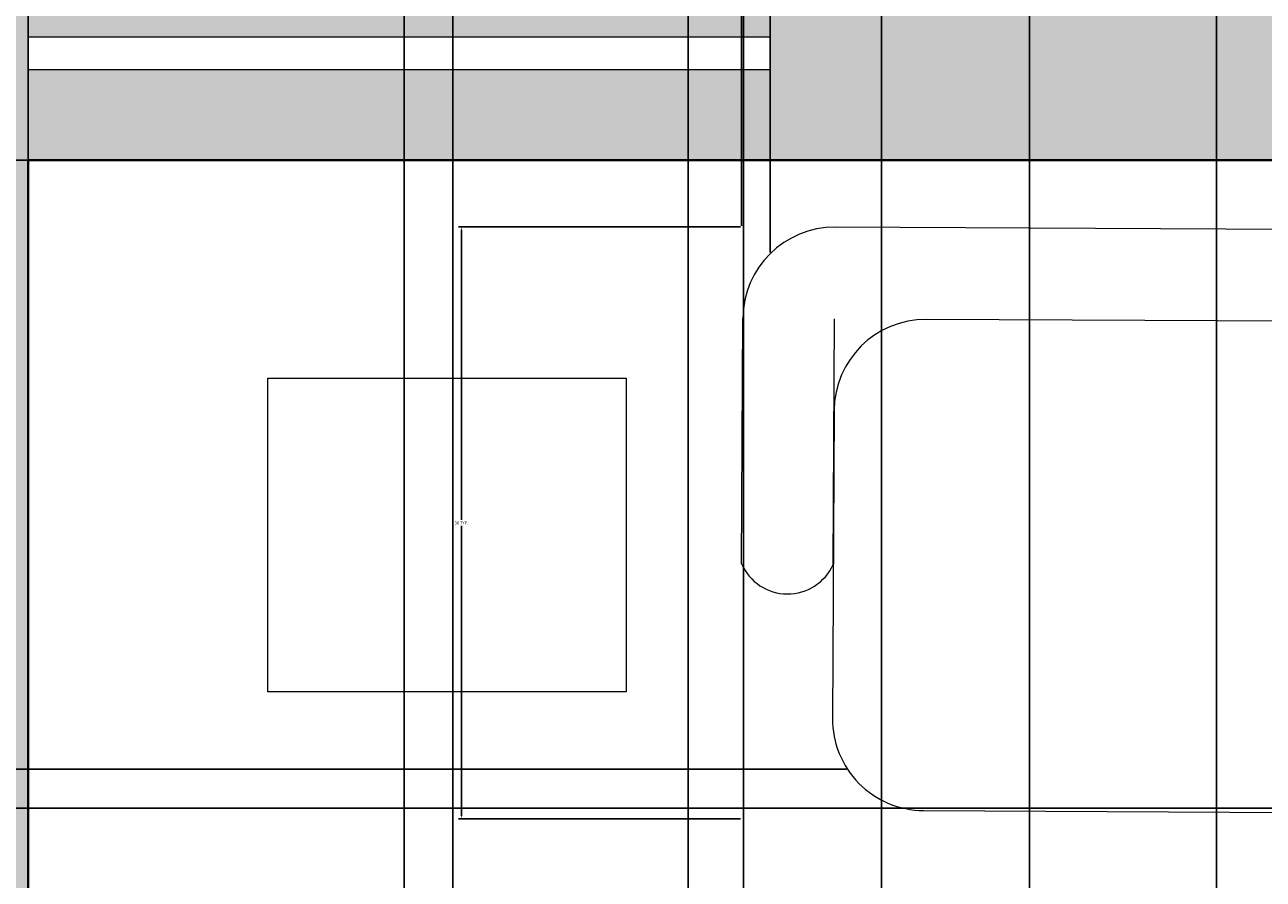
# Model space of a CAD drawing. Units: inches. Extents: x 818 to 1898, y 976 to 2364.
# Tile 28 of 96: x 1207 to 1282, y 1643 to 1695. Entities that reach past the tile are written whole.
import ezdxf

# ---------------------------------------------------------------- set-up
doc = ezdxf.new("R2010")
doc.units = ezdxf.units.IN
doc.header["$LTSCALE"] = 5
doc.header["$MEASUREMENT"] = 0
for name, color, linetype, lineweight in [('A-ANNO-DIMS', 2, 'Continuous', 18), ('A-FURN', 8, 'Continuous', 18), ('A-GLAZ', 4, 'Continuous', 18), ('A-WALL', 7, 'Continuous', 40)]:
    doc.layers.add(name, color=color, linetype=linetype, lineweight=lineweight)
doc.layers.add('A-GLAZ-PATT', color=141, linetype='Continuous', lineweight=9, true_color=0xadddf7)
doc.layers.add('A-WALL-PATT', color=251, linetype='Continuous', lineweight=13, true_color=0x636466)
doc.styles.get("Standard").update_dxf_attribs({"font": 'arial.ttf'})
doc.dimstyles.get("Standard").update_dxf_attribs({"dimtxt": 0.18, "dimasz": 0.18, "dimexe": 0.18, "dimexo": 0.0625, "dimgap": 0.09, "dimtad": 0, "dimtih": 1, "dimtoh": 1, "dimdec": 4, "dimzin": 0, "dimdsep": 46, "dimtxsty": 'Standard', "dimcen": 0.09, "dimadec": 0, "dimazin": 0, "dimtfac": 1, "dimtdec": 4, "dimtofl": 0, "dimtmove": 0, "dimatfit": 3, "dimfxl": 1, "dimtolj": 1, "dimtzin": 0, "dimarcsym": 0})

# ---------------------------------------------------------------- blocks, each defined once
blk = doc.blocks.new('SOFA-3-SEAT')
for p, q in [((39.87, 35.861), (5.697, 36.046)), ((0, 15.523), (0.081, 30.49)), ((5.586, 15.492), (5.667, 30.46)), ((34.253, 30.305), (11.253, 30.43)), ((5.637, 24.874), (5.535, 6.111)), ((11.091, 0.495), (34.091, 0.37))]:
    blk.add_line(p, q)
for centre, radius, start, end in [((5.667, 30.46), 5.586, 89.68982, 179.68982), ((11.223, 24.843), 5.586, 89.68982, 179.68982), ((2.8, 16.752), 3.058, 203.70988, 335.66977), ((11.121, 6.081), 5.586, 179.68982, 269.68982)]:
    blk.add_arc(centre, radius, start, end)
blk = doc.blocks.new('SIDE-TABLE')
blk.add_lwpolyline([(0, 19.125), (21.823, 19.125), (21.823, 0), (0, 0)], close=True)
blk = doc.blocks.new('*D42')
at = {"layer": 'A-ANNO-DIMS', "color": 0, "lineweight": -2, "ltscale": 5, "transparency": 16777216}
for p, q in [((1250.195, 1683.07), (1250.195, 1700.259)), ((1250.375, 1700.079), (1306.123, 1700.079)), ((1363.82, 1700.079), (1308.072, 1700.079)), ((1364, 1683.07), (1364, 1700.259))]:
    blk.add_line(p, q, dxfattribs=at)
at = {"layer": 'A-ANNO-DIMS', "color": 0, "ltscale": 5, "transparency": 16777216}
for points in [[(1250.375, 1700.109), (1250.375, 1700.049), (1250.195, 1700.079)], [(1363.82, 1700.109), (1363.82, 1700.049), (1364, 1700.079)]]:
    blk.add_solid(points, dxfattribs=at)
at = {"layer": 'Defpoints', "color": 0, "ltscale": 5, "transparency": 16777216}
for p in [(1364, 1700.079), (1250.195, 1683.008), (1364, 1683.008)]:
    blk.add_point(p, dxfattribs=at)
at = {"layer": 'A-ANNO-DIMS', "color": 0, "ltscale": 5, "transparency": 16777216, "insert": (1307.097, 1700.079), "char_height": 0.18, "attachment_point": 5}
blk.add_mtext('\\A1;SOFA 114 TYP.', dxfattribs=at)
blk = doc.blocks.new('*D43')
at = {"layer": 'A-ANNO-DIMS', "color": 0, "lineweight": -2, "ltscale": 5, "transparency": 16777216}
for p, q in [((1250.132, 1683.008), (1232.944, 1683.008)), ((1233.124, 1682.828), (1233.124, 1665.15)), ((1233.124, 1647.108), (1233.124, 1664.786)), ((1250.132, 1646.928), (1232.944, 1646.928))]:
    blk.add_line(p, q, dxfattribs=at)
at = {"layer": 'A-ANNO-DIMS', "color": 0, "ltscale": 5, "transparency": 16777216}
for points in [[(1233.094, 1682.828), (1233.154, 1682.828), (1233.124, 1683.008)], [(1233.094, 1647.108), (1233.154, 1647.108), (1233.124, 1646.928)]]:
    blk.add_solid(points, dxfattribs=at)
at = {"layer": 'Defpoints', "color": 0, "ltscale": 5, "transparency": 16777216}
for p in [(1233.124, 1683.008), (1250.195, 1683.008), (1250.195, 1646.928)]:
    blk.add_point(p, dxfattribs=at)
at = {"layer": 'A-ANNO-DIMS', "color": 0, "ltscale": 5, "transparency": 16777216, "insert": (1233.124, 1664.968), "char_height": 0.18, "attachment_point": 5}
blk.add_mtext('\\A1;36 TYP.', dxfattribs=at)
blk = doc.blocks.new('*D59')
at = {"layer": 'A-ANNO-DIMS', "color": 0, "lineweight": -2, "ltscale": 5, "transparency": 16777216}
for p, q in [((1251.643, 2300.393), (818.026, 2300.393)), ((818.206, 2300.213), (818.206, 1669.95)), ((818.206, 1039.323), (818.206, 1669.586)), ((896.051, 1039.143), (818.026, 1039.143))]:
    blk.add_line(p, q, dxfattribs=at)
at = {"layer": 'A-ANNO-DIMS', "color": 0, "ltscale": 5, "transparency": 16777216}
for points in [[(818.176, 2300.213), (818.236, 2300.213), (818.206, 2300.393)], [(818.176, 1039.323), (818.236, 1039.323), (818.206, 1039.143)]]:
    blk.add_solid(points, dxfattribs=at)
at = {"layer": 'Defpoints', "color": 0, "ltscale": 5, "transparency": 16777216}
for p in [(818.206, 2300.393), (1251.706, 2300.393), (896.114, 1039.143)]:
    blk.add_point(p, dxfattribs=at)
at = {"layer": 'A-ANNO-DIMS', "color": 0, "ltscale": 5, "transparency": 16777216, "insert": (818.206, 1669.768), "char_height": 0.18, "attachment_point": 5}
blk.add_mtext('\\A1;1261.2', dxfattribs=at)
blk = doc.blocks.new('*D61')
at = {"layer": 'A-ANNO-DIMS', "color": 0, "lineweight": -2, "ltscale": 5, "transparency": 16777216}
for p, q in [((1071.725, 1203.027), (1071.725, 2363.873)), ((1430.725, 1203.027), (1430.725, 2363.873)), ((1071.905, 2363.693), (1250.936, 2363.693)), ((1430.545, 2363.693), (1251.514, 2363.693))]:
    blk.add_line(p, q, dxfattribs=at)
at = {"layer": 'A-ANNO-DIMS', "color": 0, "ltscale": 5, "transparency": 16777216}
for points in [[(1071.905, 2363.723), (1071.905, 2363.663), (1071.725, 2363.693)], [(1430.545, 2363.723), (1430.545, 2363.663), (1430.725, 2363.693)]]:
    blk.add_solid(points, dxfattribs=at)
at = {"layer": 'Defpoints', "color": 0, "ltscale": 5, "transparency": 16777216}
for p in [(1430.725, 2363.693), (1071.725, 1202.964), (1430.725, 1202.964)]:
    blk.add_point(p, dxfattribs=at)
at = {"layer": 'A-ANNO-DIMS', "color": 0, "ltscale": 5, "transparency": 16777216, "insert": (1251.225, 2363.693), "char_height": 0.18, "attachment_point": 5}
blk.add_mtext('\\A1;359', dxfattribs=at)
blk = doc.blocks.new('*D64')
at = {"layer": 'A-ANNO-DIMS', "color": 0, "lineweight": -2, "ltscale": 5, "transparency": 16777216}
for p, q in [((1197.725, 1501.141), (1197.725, 2363.873)), ((1430.725, 1501.141), (1430.725, 2363.873)), ((1197.905, 2363.693), (1313.935, 2363.693)), ((1430.545, 2363.693), (1314.516, 2363.693))]:
    blk.add_line(p, q, dxfattribs=at)
at = {"layer": 'A-ANNO-DIMS', "color": 0, "ltscale": 5, "transparency": 16777216}
for points in [[(1197.905, 2363.723), (1197.905, 2363.663), (1197.725, 2363.693)], [(1430.545, 2363.723), (1430.545, 2363.663), (1430.725, 2363.693)]]:
    blk.add_solid(points, dxfattribs=at)
at = {"layer": 'Defpoints', "color": 0, "ltscale": 5, "transparency": 16777216}
for p in [(1430.725, 2363.693), (1197.725, 1501.078), (1430.725, 1501.078)]:
    blk.add_point(p, dxfattribs=at)
at = {"layer": 'A-ANNO-DIMS', "color": 0, "ltscale": 5, "transparency": 16777216, "insert": (1314.225, 2363.693), "char_height": 0.18, "attachment_point": 5}
blk.add_mtext('\\A1;233', dxfattribs=at)
blk = doc.blocks.new('*D95')
at = {"layer": 'A-ANNO-DIMS', "color": 0, "lineweight": -2, "ltscale": 5, "transparency": 16777216}
for p, q in [((1173.542, 1071.118), (1173.542, 2363.873)), ((1229.647, 1071.118), (1229.647, 2363.873)), ((1173.722, 2363.693), (1201.288, 2363.693)), ((1229.467, 2363.693), (1201.901, 2363.693))]:
    blk.add_line(p, q, dxfattribs=at)
at = {"layer": 'A-ANNO-DIMS', "color": 0, "ltscale": 5, "transparency": 16777216}
for points in [[(1173.722, 2363.723), (1173.722, 2363.663), (1173.542, 2363.693)], [(1229.467, 2363.723), (1229.467, 2363.663), (1229.647, 2363.693)]]:
    blk.add_solid(points, dxfattribs=at)
at = {"layer": 'Defpoints', "color": 0, "ltscale": 5, "transparency": 16777216}
for p in [(1229.647, 2363.693), (1173.542, 1071.055), (1229.647, 1071.055)]:
    blk.add_point(p, dxfattribs=at)
at = {"layer": 'A-ANNO-DIMS', "color": 0, "ltscale": 5, "transparency": 16777216, "insert": (1201.595, 2363.693), "char_height": 0.18, "attachment_point": 5}
blk.add_mtext('\\A1;56.1', dxfattribs=at)
blk = doc.blocks.new('*D96')
at = {"layer": 'A-ANNO-DIMS', "color": 0, "lineweight": -2, "ltscale": 5, "transparency": 16777216}
for p, q in [((1229.647, 1071.118), (1229.647, 2363.873)), ((1284.17, 1071.118), (1284.17, 2363.873)), ((1229.827, 2363.693), (1256.516, 2363.693)), ((1283.99, 2363.693), (1257.301, 2363.693))]:
    blk.add_line(p, q, dxfattribs=at)
at = {"layer": 'A-ANNO-DIMS', "color": 0, "ltscale": 5, "transparency": 16777216}
for points in [[(1229.827, 2363.723), (1229.827, 2363.663), (1229.647, 2363.693)], [(1283.99, 2363.723), (1283.99, 2363.663), (1284.17, 2363.693)]]:
    blk.add_solid(points, dxfattribs=at)
at = {"layer": 'Defpoints', "color": 0, "ltscale": 5, "transparency": 16777216}
for p in [(1284.17, 2363.693), (1229.647, 1071.055), (1284.17, 1071.055)]:
    blk.add_point(p, dxfattribs=at)
at = {"layer": 'A-ANNO-DIMS', "color": 0, "ltscale": 5, "transparency": 16777216, "insert": (1256.909, 2363.693), "char_height": 0.18, "attachment_point": 5}
blk.add_mtext('\\A1;54.52', dxfattribs=at)
blk = doc.blocks.new('*D119')
at = {"layer": 'A-ANNO-DIMS', "color": 0, "lineweight": -2, "ltscale": 5, "transparency": 16777216}
for p, q in [((1766.29, 1716.987), (818.026, 1716.987)), ((818.206, 1716.807), (818.206, 1672.428)), ((818.206, 1627.685), (818.206, 1672.064)), ((1766.29, 1627.505), (818.026, 1627.505))]:
    blk.add_line(p, q, dxfattribs=at)
at = {"layer": 'A-ANNO-DIMS', "color": 0, "ltscale": 5, "transparency": 16777216}
for points in [[(818.176, 1716.807), (818.236, 1716.807), (818.206, 1716.987)], [(818.176, 1627.685), (818.236, 1627.685), (818.206, 1627.505)]]:
    blk.add_solid(points, dxfattribs=at)
at = {"layer": 'Defpoints', "color": 0, "ltscale": 5, "transparency": 16777216}
for p in [(818.206, 1716.987), (1766.352, 1716.987), (1766.352, 1627.505)]:
    blk.add_point(p, dxfattribs=at)
at = {"layer": 'A-ANNO-DIMS', "color": 0, "ltscale": 5, "transparency": 16777216, "insert": (818.206, 1672.246), "char_height": 0.18, "attachment_point": 5}
blk.add_mtext('\\A1;89.48', dxfattribs=at)
blk = doc.blocks.new('*D145')
at = {"layer": 'A-ANNO-DIMS', "color": 0, "lineweight": -2, "ltscale": 5, "transparency": 16777216}
for p, q in [((1197.393, 2122.314), (1197.393, 975.663)), ((1232.609, 2122.314), (1232.609, 975.663)), ((1197.573, 975.843), (1214.608, 975.843)), ((1232.429, 975.843), (1215.394, 975.843))]:
    blk.add_line(p, q, dxfattribs=at)
at = {"layer": 'A-ANNO-DIMS', "color": 0, "ltscale": 5, "transparency": 16777216}
for points in [[(1197.573, 975.873), (1197.573, 975.813), (1197.393, 975.843)], [(1232.429, 975.873), (1232.429, 975.813), (1232.609, 975.843)]]:
    blk.add_solid(points, dxfattribs=at)
at = {"layer": 'Defpoints', "color": 0, "ltscale": 5, "transparency": 16777216}
for p in [(1197.393, 2122.377), (1232.609, 2122.377), (1232.609, 975.843)]:
    blk.add_point(p, dxfattribs=at)
at = {"layer": 'A-ANNO-DIMS', "color": 0, "ltscale": 5, "transparency": 16777216, "insert": (1215.001, 975.843), "char_height": 0.18, "attachment_point": 5}
blk.add_mtext('\\A1;35.22', dxfattribs=at)
blk = doc.blocks.new('*D159')
at = {"layer": 'A-ANNO-DIMS', "color": 0, "lineweight": -2, "ltscale": 5, "transparency": 16777216}
for p, q in [((1206.725, 1687.016), (1206.725, 975.663)), ((1463.725, 1687.016), (1463.725, 975.663)), ((1206.905, 975.843), (1334.935, 975.843)), ((1463.545, 975.843), (1335.516, 975.843))]:
    blk.add_line(p, q, dxfattribs=at)
at = {"layer": 'A-ANNO-DIMS', "color": 0, "ltscale": 5, "transparency": 16777216}
for points in [[(1206.905, 975.873), (1206.905, 975.813), (1206.725, 975.843)], [(1463.545, 975.873), (1463.545, 975.813), (1463.725, 975.843)]]:
    blk.add_solid(points, dxfattribs=at)
at = {"layer": 'Defpoints', "color": 0, "ltscale": 5, "transparency": 16777216}
for p in [(1206.725, 1687.078), (1463.725, 1687.078), (1463.725, 975.843)]:
    blk.add_point(p, dxfattribs=at)
at = {"layer": 'A-ANNO-DIMS', "color": 0, "ltscale": 5, "transparency": 16777216, "insert": (1335.225, 975.843), "char_height": 0.18, "attachment_point": 5}
blk.add_mtext('\\A1;257', dxfattribs=at)
blk = doc.blocks.new('*D176')
at = {"layer": 'A-ANNO-DIMS', "color": 0, "lineweight": -2, "ltscale": 5, "transparency": 16777216}
for p, q in [((1559.663, 1687.078), (818.026, 1687.078)), ((818.206, 1686.898), (818.206, 1667.51)), ((818.206, 1647.758), (818.206, 1667.146)), ((1559.663, 1647.578), (818.026, 1647.578))]:
    blk.add_line(p, q, dxfattribs=at)
at = {"layer": 'A-ANNO-DIMS', "color": 0, "ltscale": 5, "transparency": 16777216}
for points in [[(818.176, 1686.898), (818.236, 1686.898), (818.206, 1687.078)], [(818.176, 1647.758), (818.236, 1647.758), (818.206, 1647.578)]]:
    blk.add_solid(points, dxfattribs=at)
at = {"layer": 'Defpoints', "color": 0, "ltscale": 5, "transparency": 16777216}
for p in [(1559.725, 1687.078), (818.206, 1647.578), (1559.725, 1647.578)]:
    blk.add_point(p, dxfattribs=at)
at = {"layer": 'A-ANNO-DIMS', "color": 0, "ltscale": 5, "transparency": 16777216, "insert": (818.206, 1667.328), "char_height": 0.18, "attachment_point": 5}
blk.add_mtext('\\A1;39.5', dxfattribs=at)
blk = doc.blocks.new('*D215')
at = {"layer": 'A-ANNO-DIMS', "color": 0, "lineweight": -2, "ltscale": 5, "transparency": 16777216}
for p, q in [((1590.663, 1876.078), (818.026, 1876.078)), ((818.206, 1875.898), (818.206, 1781.76)), ((818.206, 1687.258), (818.206, 1781.396)), ((1511.663, 1687.078), (818.026, 1687.078))]:
    blk.add_line(p, q, dxfattribs=at)
at = {"layer": 'A-ANNO-DIMS', "color": 0, "ltscale": 5, "transparency": 16777216}
for points in [[(818.176, 1875.898), (818.236, 1875.898), (818.206, 1876.078)], [(818.176, 1687.258), (818.236, 1687.258), (818.206, 1687.078)]]:
    blk.add_solid(points, dxfattribs=at)
at = {"layer": 'Defpoints', "color": 0, "ltscale": 5, "transparency": 16777216}
for p in [(818.206, 1876.078), (1590.725, 1876.078), (1511.725, 1687.078)]:
    blk.add_point(p, dxfattribs=at)
at = {"layer": 'A-ANNO-DIMS', "color": 0, "ltscale": 5, "transparency": 16777216, "insert": (818.206, 1781.578), "char_height": 0.18, "attachment_point": 5}
blk.add_mtext('\\A1;189', dxfattribs=at)
blk = doc.blocks.new('*D233')
at = {"layer": 'A-ANNO-DIMS', "color": 0, "lineweight": -2, "ltscale": 5, "transparency": 16777216}
for p, q in [((1267.725, 2044.016), (1267.725, 975.663)), ((1303.931, 2008.329), (1303.931, 975.663)), ((1267.905, 975.843), (1285.365, 975.843)), ((1303.751, 975.843), (1286.292, 975.843))]:
    blk.add_line(p, q, dxfattribs=at)
at = {"layer": 'A-ANNO-DIMS', "color": 0, "ltscale": 5, "transparency": 16777216}
for points in [[(1267.905, 975.873), (1267.905, 975.813), (1267.725, 975.843)], [(1303.751, 975.873), (1303.751, 975.813), (1303.931, 975.843)]]:
    blk.add_solid(points, dxfattribs=at)
at = {"layer": 'Defpoints', "color": 0, "ltscale": 5, "transparency": 16777216}
for p in [(1267.725, 2044.078), (1303.931, 2008.392), (1303.931, 975.843)]:
    blk.add_point(p, dxfattribs=at)
at = {"layer": 'A-ANNO-DIMS', "color": 0, "ltscale": 5, "transparency": 16777216, "insert": (1285.828, 975.843), "char_height": 0.18, "attachment_point": 5}
blk.add_mtext('\\A1;36.206', dxfattribs=at)
blk = doc.blocks.new('*D251')
at = {"layer": 'A-ANNO-DIMS', "color": 0, "lineweight": -2, "ltscale": 5, "transparency": 16777216}
for p, q in [((1250.303, 1878.329), (1250.303, 975.663)), ((1258.725, 1878.329), (1258.725, 975.663)), ((1250.483, 975.843), (1254.121, 975.843)), ((1258.545, 975.843), (1254.907, 975.843))]:
    blk.add_line(p, q, dxfattribs=at)
at = {"layer": 'A-ANNO-DIMS', "color": 0, "ltscale": 5, "transparency": 16777216}
for points in [[(1250.483, 975.873), (1250.483, 975.813), (1250.303, 975.843)], [(1258.545, 975.873), (1258.545, 975.813), (1258.725, 975.843)]]:
    blk.add_solid(points, dxfattribs=at)
at = {"layer": 'Defpoints', "color": 0, "ltscale": 5, "transparency": 16777216}
for p in [(1250.303, 1878.392), (1258.725, 1878.392), (1258.725, 975.843)]:
    blk.add_point(p, dxfattribs=at)
at = {"layer": 'A-ANNO-DIMS', "color": 0, "ltscale": 5, "transparency": 16777216, "insert": (1254.514, 975.843), "char_height": 0.18, "attachment_point": 5}
blk.add_mtext('\\A1;8.422', dxfattribs=at)
blk = doc.blocks.new('*D254')
at = {"layer": 'A-ANNO-DIMS', "color": 0, "lineweight": -2, "ltscale": 5, "transparency": 16777216}
for p, q in [((1267.725, 2044.016), (1267.725, 975.663)), ((1330.305, 2044.016), (1330.305, 975.663)), ((1267.905, 975.843), (1298.621, 975.843)), ((1330.125, 975.843), (1299.409, 975.843))]:
    blk.add_line(p, q, dxfattribs=at)
at = {"layer": 'A-ANNO-DIMS', "color": 0, "ltscale": 5, "transparency": 16777216}
for points in [[(1267.905, 975.873), (1267.905, 975.813), (1267.725, 975.843)], [(1330.125, 975.873), (1330.125, 975.813), (1330.305, 975.843)]]:
    blk.add_solid(points, dxfattribs=at)
at = {"layer": 'Defpoints', "color": 0, "ltscale": 5, "transparency": 16777216}
for p in [(1267.725, 2044.078), (1330.305, 2044.078), (1330.305, 975.843)]:
    blk.add_point(p, dxfattribs=at)
at = {"layer": 'A-ANNO-DIMS', "color": 0, "ltscale": 5, "transparency": 16777216, "insert": (1299.015, 975.843), "char_height": 0.18, "attachment_point": 5}
blk.add_mtext('\\A1;62.58', dxfattribs=at)
blk = doc.blocks.new('*D269')
at = {"layer": 'A-ANNO-DIMS', "color": 0, "lineweight": -2, "ltscale": 5, "transparency": 16777216}
for p, q in [((1246.938, 1534.141), (1246.938, 2363.873)), ((1341.259, 1534.141), (1341.259, 2363.873)), ((1247.118, 2363.693), (1293.706, 2363.693)), ((1341.079, 2363.693), (1294.491, 2363.693))]:
    blk.add_line(p, q, dxfattribs=at)
at = {"layer": 'A-ANNO-DIMS', "color": 0, "ltscale": 5, "transparency": 16777216}
for points in [[(1247.118, 2363.723), (1247.118, 2363.663), (1246.938, 2363.693)], [(1341.079, 2363.723), (1341.079, 2363.663), (1341.259, 2363.693)]]:
    blk.add_solid(points, dxfattribs=at)
at = {"layer": 'Defpoints', "color": 0, "ltscale": 5, "transparency": 16777216}
for p in [(1341.259, 2363.693), (1246.938, 1534.078), (1341.259, 1534.078)]:
    blk.add_point(p, dxfattribs=at)
at = {"layer": 'A-ANNO-DIMS', "color": 0, "ltscale": 5, "transparency": 16777216, "insert": (1294.099, 2363.693), "char_height": 0.18, "attachment_point": 5}
blk.add_mtext('\\A1;94.32', dxfattribs=at)
blk = doc.blocks.new('*D271')
at = {"layer": 'A-ANNO-DIMS', "color": 0, "lineweight": -2, "ltscale": 5, "transparency": 16777216}
for p, q in [((1206.725, 1510.141), (1206.725, 2363.873)), ((1246.938, 1510.141), (1246.938, 2363.873)), ((1206.905, 2363.693), (1226.451, 2363.693)), ((1246.758, 2363.693), (1227.211, 2363.693))]:
    blk.add_line(p, q, dxfattribs=at)
at = {"layer": 'A-ANNO-DIMS', "color": 0, "ltscale": 5, "transparency": 16777216}
for points in [[(1206.905, 2363.723), (1206.905, 2363.663), (1206.725, 2363.693)], [(1246.758, 2363.723), (1246.758, 2363.663), (1246.938, 2363.693)]]:
    blk.add_solid(points, dxfattribs=at)
at = {"layer": 'Defpoints', "color": 0, "ltscale": 5, "transparency": 16777216}
for p in [(1246.938, 2363.693), (1206.725, 1510.078), (1246.938, 1510.078)]:
    blk.add_point(p, dxfattribs=at)
at = {"layer": 'A-ANNO-DIMS', "color": 0, "ltscale": 5, "transparency": 16777216, "insert": (1226.831, 2363.693), "char_height": 0.18, "attachment_point": 5}
blk.add_mtext('\\A1;40.21', dxfattribs=at)
blk = doc.blocks.new('*D276')
at = {"layer": 'A-ANNO-DIMS', "color": 0, "lineweight": -2, "ltscale": 5, "transparency": 16777216}
for p, q in [((1206.725, 1687.141), (1206.725, 2363.873)), ((1251.933, 1681.439), (1251.933, 2363.873)), ((1206.905, 2363.693), (1228.949, 2363.693)), ((1251.753, 2363.693), (1229.709, 2363.693))]:
    blk.add_line(p, q, dxfattribs=at)
at = {"layer": 'A-ANNO-DIMS', "color": 0, "ltscale": 5, "transparency": 16777216}
for points in [[(1206.905, 2363.723), (1206.905, 2363.663), (1206.725, 2363.693)], [(1251.753, 2363.723), (1251.753, 2363.663), (1251.933, 2363.693)]]:
    blk.add_solid(points, dxfattribs=at)
at = {"layer": 'Defpoints', "color": 0, "ltscale": 5, "transparency": 16777216}
for p in [(1251.933, 2363.693), (1206.725, 1687.078), (1251.933, 1681.376)]:
    blk.add_point(p, dxfattribs=at)
at = {"layer": 'A-ANNO-DIMS', "color": 0, "ltscale": 5, "transparency": 16777216, "insert": (1229.329, 2363.693), "char_height": 0.18, "attachment_point": 5}
blk.add_mtext('\\A1;45.21', dxfattribs=at)
blk = doc.blocks.new('*D277')
at = {"layer": 'A-ANNO-DIMS', "color": 0, "lineweight": -2, "ltscale": 5, "transparency": 16777216}
for p, q in [((1251.871, 1687.078), (818.026, 1687.078)), ((818.206, 1686.898), (818.206, 1668.697)), ((818.206, 1650.132), (818.206, 1668.333)), ((1256.589, 1649.952), (818.026, 1649.952))]:
    blk.add_line(p, q, dxfattribs=at)
at = {"layer": 'A-ANNO-DIMS', "color": 0, "ltscale": 5, "transparency": 16777216}
for points in [[(818.176, 1686.898), (818.236, 1686.898), (818.206, 1687.078)], [(818.176, 1650.132), (818.236, 1650.132), (818.206, 1649.952)]]:
    blk.add_solid(points, dxfattribs=at)
at = {"layer": 'Defpoints', "color": 0, "ltscale": 5, "transparency": 16777216}
for p in [(818.206, 1687.078), (1251.933, 1687.078), (1256.652, 1649.952)]:
    blk.add_point(p, dxfattribs=at)
at = {"layer": 'A-ANNO-DIMS', "color": 0, "ltscale": 5, "transparency": 16777216, "insert": (818.206, 1668.515), "char_height": 0.18, "attachment_point": 5}
blk.add_mtext('\\A1;37.13', dxfattribs=at)
blk = doc.blocks.new('*D278')
at = {"layer": 'A-ANNO-DIMS', "color": 0, "lineweight": -2, "ltscale": 5, "transparency": 16777216}
for p, q in [((1324.033, 1700.743), (1324.033, 975.663)), ((1267.725, 1696.016), (1267.725, 975.663)), ((1267.905, 975.843), (1295.503, 975.843)), ((1323.853, 975.843), (1296.256, 975.843))]:
    blk.add_line(p, q, dxfattribs=at)
at = {"layer": 'A-ANNO-DIMS', "color": 0, "ltscale": 5, "transparency": 16777216}
for points in [[(1267.905, 975.873), (1267.905, 975.813), (1267.725, 975.843)], [(1323.853, 975.873), (1323.853, 975.813), (1324.033, 975.843)]]:
    blk.add_solid(points, dxfattribs=at)
at = {"layer": 'Defpoints', "color": 0, "ltscale": 5, "transparency": 16777216}
for p in [(1324.033, 1700.806), (1267.725, 1696.078), (1324.033, 975.843)]:
    blk.add_point(p, dxfattribs=at)
at = {"layer": 'A-ANNO-DIMS', "color": 0, "ltscale": 5, "transparency": 16777216, "insert": (1295.879, 975.843), "char_height": 0.18, "attachment_point": 5}
blk.add_mtext('\\A1;56.31', dxfattribs=at)
blk = doc.blocks.new('*D279')
at = {"layer": 'A-ANNO-DIMS', "color": 0, "lineweight": -2, "ltscale": 5, "transparency": 16777216}
for p, q in [((1279.125, 1713.755), (1279.125, 975.663)), ((1267.725, 1696.016), (1267.725, 975.663)), ((1267.905, 975.843), (1273.11, 975.843)), ((1278.945, 975.843), (1273.74, 975.843))]:
    blk.add_line(p, q, dxfattribs=at)
at = {"layer": 'A-ANNO-DIMS', "color": 0, "ltscale": 5, "transparency": 16777216}
for points in [[(1267.905, 975.873), (1267.905, 975.813), (1267.725, 975.843)], [(1278.945, 975.873), (1278.945, 975.813), (1279.125, 975.843)]]:
    blk.add_solid(points, dxfattribs=at)
at = {"layer": 'Defpoints', "color": 0, "ltscale": 5, "transparency": 16777216}
for p in [(1279.125, 1713.817), (1267.725, 1696.078), (1267.725, 975.843)]:
    blk.add_point(p, dxfattribs=at)
at = {"layer": 'A-ANNO-DIMS', "color": 0, "ltscale": 5, "transparency": 16777216, "insert": (1273.425, 975.843), "char_height": 0.18, "attachment_point": 5}
blk.add_mtext('\\A1;11.4', dxfattribs=at)
blk = doc.blocks.new('*D283')
at = {"layer": 'A-ANNO-DIMS', "color": 0, "lineweight": -2, "ltscale": 5, "transparency": 16777216}
for p, q in [((1351.599, 1761.386), (1351.599, 975.663)), ((1267.725, 1696.016), (1267.725, 975.663)), ((1267.905, 975.843), (1309.268, 975.843)), ((1351.419, 975.843), (1310.056, 975.843))]:
    blk.add_line(p, q, dxfattribs=at)
at = {"layer": 'A-ANNO-DIMS', "color": 0, "ltscale": 5, "transparency": 16777216}
for points in [[(1267.905, 975.873), (1267.905, 975.813), (1267.725, 975.843)], [(1351.419, 975.873), (1351.419, 975.813), (1351.599, 975.843)]]:
    blk.add_solid(points, dxfattribs=at)
at = {"layer": 'Defpoints', "color": 0, "ltscale": 5, "transparency": 16777216}
for p in [(1351.599, 1761.449), (1267.725, 1696.078), (1351.599, 975.843)]:
    blk.add_point(p, dxfattribs=at)
at = {"layer": 'A-ANNO-DIMS', "color": 0, "ltscale": 5, "transparency": 16777216, "insert": (1309.662, 975.843), "char_height": 0.18, "attachment_point": 5}
blk.add_mtext('\\A1;83.87', dxfattribs=at)
blk = doc.blocks.new('*D285')
at = {"layer": 'A-ANNO-DIMS', "color": 0, "lineweight": -2, "ltscale": 5, "transparency": 16777216}
for p, q in [((1305.828, 1830.022), (1305.828, 975.663)), ((1267.725, 1814.903), (1267.725, 975.663)), ((1267.905, 975.843), (1286.47, 975.843)), ((1305.648, 975.843), (1287.083, 975.843))]:
    blk.add_line(p, q, dxfattribs=at)
at = {"layer": 'A-ANNO-DIMS', "color": 0, "ltscale": 5, "transparency": 16777216}
for points in [[(1267.905, 975.873), (1267.905, 975.813), (1267.725, 975.843)], [(1305.648, 975.873), (1305.648, 975.813), (1305.828, 975.843)]]:
    blk.add_solid(points, dxfattribs=at)
at = {"layer": 'Defpoints', "color": 0, "ltscale": 5, "transparency": 16777216}
for p in [(1305.828, 1830.084), (1267.725, 1814.965), (1267.725, 975.843)]:
    blk.add_point(p, dxfattribs=at)
at = {"layer": 'A-ANNO-DIMS', "color": 0, "ltscale": 5, "transparency": 16777216, "insert": (1286.776, 975.843), "char_height": 0.18, "attachment_point": 5}
blk.add_mtext('\\A1;38.1', dxfattribs=at)
blk = doc.blocks.new('*D291')
at = {"layer": 'A-ANNO-DIMS', "color": 0, "lineweight": -2, "ltscale": 5, "transparency": 16777216}
for p, q in [((1206.788, 1687.078), (1897.916, 1687.078)), ((1897.736, 1686.898), (1897.736, 1647.606)), ((1897.736, 1607.951), (1897.736, 1647.242)), ((1318.956, 1607.771), (1897.916, 1607.771))]:
    blk.add_line(p, q, dxfattribs=at)
at = {"layer": 'A-ANNO-DIMS', "color": 0, "ltscale": 5, "transparency": 16777216}
for points in [[(1897.706, 1686.898), (1897.766, 1686.898), (1897.736, 1687.078)], [(1897.706, 1607.951), (1897.766, 1607.951), (1897.736, 1607.771)]]:
    blk.add_solid(points, dxfattribs=at)
at = {"layer": 'Defpoints', "color": 0, "ltscale": 5, "transparency": 16777216}
for p in [(1206.725, 1687.078), (1897.736, 1687.078), (1318.893, 1607.771)]:
    blk.add_point(p, dxfattribs=at)
at = {"layer": 'A-ANNO-DIMS', "color": 0, "ltscale": 5, "transparency": 16777216, "insert": (1897.736, 1647.424), "char_height": 0.18, "attachment_point": 5}
blk.add_mtext('\\A1;79.3', dxfattribs=at)

msp = doc.modelspace()

# ---------------------------------------------------------------- hatches: boundary and pattern name
at = {"layer": 'A-GLAZ-PATT', "ltscale": 5}
h = msp.add_hatch(color=256, dxfattribs=at)
h.dxf.hatch_style = 1
h.paths.add_polyline_path([(1283.8183, 1504.5782), (1206.7251, 1504.5782), (1206.7251, 1501.0782), (1283.8183, 1501.0782)])
h.paths.add_polyline_path([(1283.8183, 1510.0782), (1206.7251, 1510.0782), (1206.7251, 1506.5782), (1283.8183, 1506.5782)])
h.paths.add_polyline_path([(1490.9163, 1355.0782), (1439.7252, 1355.0782), (1439.7252, 1409.0522), (1436.2252, 1409.0522), (1436.2252, 1351.5782), (1490.9163, 1351.5782)])
h.paths.add_polyline_path([(1434.2252, 1409.0522), (1430.7251, 1409.0522), (1430.7251, 1346.0782), (1435.0799, 1346.0782), (1435.0731, 1346.1152), (1435.1501, 1346.0782), (1490.9163, 1346.0782), (1490.9163, 1349.5782), (1434.2252, 1349.5782)])
h.paths.add_polyline_path([(1714.7252, 1545.0782), (1711.2252, 1545.0782), (1711.2252, 1521.0782), (1714.7252, 1521.0782)])
h.paths.add_polyline_path([(1709.2252, 1545.0782), (1705.7252, 1545.0782), (1705.7252, 1521.0782), (1709.2252, 1521.0782)])
h.paths.add_polyline_path([(1714.7252, 1687.0782), (1711.2252, 1687.0782), (1711.2252, 1649.9029), (1714.7252, 1649.9029)])
h.paths.add_polyline_path([(1709.2252, 1687.0782), (1705.7252, 1687.0782), (1705.7252, 1649.9029), (1709.2252, 1649.9029)])
h.paths.add_polyline_path([(1709.2252, 1745.5584), (1705.7252, 1745.5584), (1705.7252, 1717.3178), (1709.2252, 1717.3178)])
h.paths.add_polyline_path([(1714.7252, 1745.5584), (1711.2252, 1745.5584), (1711.2252, 1717.3178), (1714.7252, 1717.3178)])
h.paths.add_polyline_path([(1714.7252, 2014.5114), (1711.2252, 2014.5114), (1711.2252, 1962.0338), (1714.7252, 1962.0338)])
h.paths.add_polyline_path([(1709.2252, 2014.5114), (1705.7252, 2014.5114), (1705.7252, 1962.0338), (1709.2252, 1962.0338)])
h.paths.add_polyline_path([(1538.5155, 2047.5782), (1485.1216, 2047.5782), (1485.1216, 2044.0782), (1538.5155, 2044.0782)])
h.paths.add_polyline_path([(1538.5155, 2053.0782), (1485.1216, 2053.0782), (1485.1216, 2049.5782), (1538.5155, 2049.5782)])
h.paths.add_polyline_path([(1388.0315, 2047.5782), (1330.305, 2047.5782), (1330.305, 2044.0782), (1388.0315, 2044.0782)])
h.paths.add_polyline_path([(1388.0315, 2053.0782), (1330.305, 2053.0782), (1330.305, 2049.5782), (1388.0315, 2049.5782)])
h.paths.add_polyline_path([(1262.2252, 2019.2871), (1258.7251, 2019.2871), (1258.7251, 1928.9218), (1262.2252, 1928.9218)])
h.paths.add_polyline_path([(1267.7251, 2019.2871), (1264.2252, 2019.2871), (1264.2252, 1928.9218), (1267.7251, 1928.9218)])
h.paths.add_polyline_path([(1262.2252, 1862.9652), (1258.7251, 1862.9652), (1258.7251, 1814.9652), (1262.2252, 1814.9652)])
h.paths.add_polyline_path([(1267.7251, 1862.9652), (1264.2252, 1862.9652), (1264.2252, 1814.9652), (1267.7251, 1814.9652)])
h.paths.add_polyline_path([(1262.2252, 1755.3321), (1258.7251, 1755.3321), (1258.7251, 1707.3321), (1262.2252, 1707.3321)])
h.paths.add_polyline_path([(1267.7251, 1755.3321), (1264.2252, 1755.3321), (1264.2252, 1707.3321), (1267.7251, 1707.3321)])
h.paths.add_polyline_path([(1251.9333, 1692.5782), (1206.7251, 1692.5782), (1206.7251, 1687.0782), (1251.9333, 1687.0782)])
h.paths.add_polyline_path([(1251.9333, 1700.0782), (1206.7251, 1700.0782), (1206.7251, 1694.5782), (1251.9333, 1694.5782)])
at = {"layer": 'A-WALL-PATT', "ltscale": 5}
h = msp.add_hatch(color=256, dxfattribs=at)
h.dxf.hatch_style = 1
h.paths.add_polyline_path([(1267.7251, 1928.9218), (1258.7251, 1928.9218), (1258.7251, 1913.6401), (1250.3029, 1913.6401), (1250.3029, 1878.3919), (1258.7251, 1878.3919), (1258.7251, 1862.9652), (1267.7251, 1862.9652)])
h.paths.add_polyline_path([(1267.7251, 1814.9652), (1258.7251, 1814.9652), (1258.7251, 1755.3321), (1267.7251, 1755.3321)])
h.paths.add_polyline_path([(1463.7251, 1696.0782), (1267.7251, 1696.0782), (1267.7251, 1707.3321), (1258.7251, 1707.3321), (1258.7251, 1700.0782), (1251.9333, 1700.0782), (1251.9333, 1687.0782), (1463.7251, 1687.0782)])
h.paths.add_polyline_path([(1714.7252, 1717.3178), (1705.7252, 1717.3178), (1705.7252, 1696.0782), (1599.7252, 1696.0782), (1599.7252, 1790.0782), (1705.7252, 1790.0782), (1705.7252, 1785.6125), (1714.7252, 1785.6125), (1714.7252, 1827.2125), (1705.7252, 1827.2125), (1705.7252, 1802.0782), (1599.7252, 1802.0782), (1599.7252, 1867.0782), (1705.7252, 1867.0782), (1705.7252, 1857.2125), (1714.7252, 1857.2125), (1714.7252, 1930.0316), (1741.8409, 1930.0316), (1741.8409, 1935.0316), (1714.7252, 1935.0316), (1714.7252, 1957.0338), (1741.8409, 1957.0338), (1741.8409, 1962.0338), (1714.7252, 1962.0338), (1705.7252, 1962.0338), (1705.7252, 1948.0782), (1599.7252, 1948.0782), (1599.7252, 1981.0782), (1590.7251, 1981.0782), (1590.7251, 1941.0782), (1620.7252, 1941.0782), (1705.7252, 1941.0782), (1705.7252, 1876.0782), (1599.7252, 1876.0782), (1599.7252, 1911.0782), (1590.7251, 1911.0782), (1590.7251, 1876.0782), (1429.2252, 1876.0782), (1429.2252, 1867.0782), (1511.7251, 1867.0782), (1528.593, 1867.0782), (1595.7252, 1867.0782), (1595.7252, 1773.0782), (1520.7252, 1773.0782), (1520.7252, 1837.5823), (1532.593, 1837.5823), (1532.593, 1867.0782), (1528.593, 1867.0782), (1528.593, 1841.5823), (1511.7251, 1841.5823), (1511.7251, 1744.9714), (1520.7252, 1744.9714), (1520.7252, 1761.0782), (1595.7252, 1761.0782), (1595.7252, 1696.0782), (1520.7252, 1696.0782), (1520.7252, 1716.0454), (1511.7251, 1716.0454), (1511.7251, 1696.0782), (1511.7251, 1687.0782), (1714.7252, 1687.0782)])
h.paths.add_polyline_path([(1714.7252, 2053.0782), (1714.7252, 2081.1881), (1709.7252, 2081.1881), (1709.7252, 2053.0782), (1681.6446, 2053.0782), (1681.6446, 2081.1881), (1676.6446, 2081.1881), (1676.6446, 2053.0782), (1538.5155, 2053.0782), (1538.5155, 2044.0782), (1590.7251, 2044.0782), (1590.7251, 2011.0782), (1599.7252, 2011.0782), (1599.7252, 2044.0782), (1705.7252, 2044.0782), (1705.7252, 2014.5114), (1714.7252, 2014.5114)])
h.paths.add_polyline_path([(1485.1216, 2053.0782), (1422.02, 2053.0782), (1422.02, 2081.1881), (1413.02, 2081.1881), (1413.02, 2053.0782), (1399.6356, 2053.0782), (1399.6356, 2081.1881), (1390.6356, 2081.1881), (1390.6356, 2053.0782), (1388.0315, 2053.0782), (1388.0315, 2044.0782), (1416.2743, 2044.0782), (1485.1216, 2044.0782)])
h.paths.add_polyline_path([(1330.305, 2053.0782), (1258.7251, 2053.0782), (1258.7251, 2019.2871), (1267.7251, 2019.2871), (1267.7251, 2044.0782), (1330.305, 2044.0782)])
h.paths.add_polyline_path([(1258.7251, 2053.0782), (1214.6577, 2053.0782), (1214.6577, 2044.0782), (1258.7251, 2044.0782)])
h.paths.add_polyline_path([(1214.6577, 2053.0782), (1180.349, 2053.0782), (1180.349, 2044.0782), (1214.6577, 2044.0782)])
h.paths.add_polyline_path([(1714.7252, 1639.5782), (1741.8409, 1639.5782), (1741.8409, 1643.5782), (1714.7252, 1643.5782), (1714.7252, 1649.9029), (1705.7252, 1649.9029), (1705.7252, 1600.0782), (1477.7252, 1600.0782), (1477.7252, 1591.0782), (1520.7252, 1591.0782), (1616.7252, 1591.0782), (1616.7252, 1416.6857), (1622.7252, 1416.6857), (1622.7252, 1463.0782), (1624.7252, 1463.0782), (1624.7252, 1467.0782), (1622.7252, 1467.0782), (1622.7252, 1591.0782), (1705.7252, 1591.0782), (1705.7252, 1545.0782), (1714.7252, 1545.0782), (1741.8409, 1545.0782), (1741.8409, 1549.0782), (1714.7252, 1549.0782), (1714.7252, 1593.9175), (1737.8409, 1593.9175), (1737.8409, 1597.9175), (1714.7252, 1597.9175)])
h.paths.add_polyline_path([(1674.9024, 2060.7419), (1714.7045, 2060.7419), (1714.7045, 2073.1061), (1674.9024, 2073.1061)], flags=25)
h.paths.add_polyline_path([(1394.5468, 2061.6618), (1422.2344, 2061.6618), (1422.2344, 2074.0261), (1394.5468, 2074.0261)], flags=24)
h = msp.add_hatch(color=256, dxfattribs=at)
h.dxf.hatch_style = 1
h.paths.add_polyline_path([(1206.7251, 1687.0782), (1206.7251, 1700.0782), (1197.7251, 1700.0782), (1197.7251, 1501.0782), (1206.7251, 1501.0782), (1206.7251, 1510.0782)])
h.paths.add_polyline_path([(1197.7251, 1590.7585), (1173.7252, 1590.7585), (1173.7252, 1586.7585), (1197.7251, 1586.7585)])
h.paths.add_polyline_path([(1197.7251, 1534.6024), (1173.7252, 1534.6024), (1173.7252, 1530.6024), (1197.7251, 1530.6024)])
h.paths.add_polyline_path([(1365.1463, 1510.0782), (1283.8183, 1510.0782), (1283.8183, 1501.0782), (1365.1463, 1501.0782)])
h.paths.add_polyline_path([(1439.7252, 1591.0782), (1441.7252, 1591.0782), (1441.7252, 1600.0782), (1430.7251, 1600.0782), (1430.7251, 1510.0782), (1406.7252, 1510.0782), (1401.1463, 1510.0782), (1401.1463, 1501.0782), (1430.7251, 1501.0782), (1430.7251, 1486.2383), (1430.7251, 1409.0522), (1439.7252, 1409.0522)])

# ---------------------------------------------------------------- linework, layer by layer
at = {"layer": 'A-GLAZ'}
for p, q in [((1206.7251, 1687.0782), (1206.7251, 1700.0782)), ((1251.9333, 1700.0782), (1251.9333, 1687.0782))]:
    msp.add_line(p, q, dxfattribs=at)
at = {"layer": 'A-GLAZ', "ltscale": 5}
for p, q in [((1251.9333, 1694.5782), (1206.7251, 1694.5782)), ((1251.9333, 1692.5782), (1206.7251, 1692.5782))]:
    msp.add_line(p, q, dxfattribs=at)
at = {"layer": 'A-WALL'}
for q in [(1463.7251, 1687.0782), (1206.7251, 1510.0782)]:
    msp.add_line((1206.7251, 1687.0782), q, dxfattribs=at)

# ---------------------------------------------------------------- block references
at = {"layer": 'A-FURN'}
for name, p in [('SOFA-3-SEAT', (1250.195, 1646.945)), ('SIDE-TABLE', (1221.338, 1654.674))]:
    msp.add_blockref(name, p, dxfattribs=at)

# ---------------------------------------------------------------- dimensions: what is measured, and where the dimension line sits
at = {"layer": 'A-ANNO-DIMS', "ltscale": 5}
for base, p1, p2, override, picture, middle in [((1430.7251, 2363.6929), (1071.7251, 1202.9642), (1430.7251, 1202.9642), {"dimdec": 0, "dimlfac": 1, "dimrnd": 0, "dimzin": 0, "dimdsep": 46, "dimlunit": 2}, '*D61', (1251.2251, 2363.6929)), ((1229.6474, 2363.6929), (1173.5418, 1071.0552), (1229.6474, 1071.0552), {"dimdec": 1, "dimlfac": 1, "dimrnd": 0, "dimzin": 0, "dimdsep": 46, "dimlunit": 2}, '*D95', (1201.5946, 2363.6929)), ((1430.7251, 2363.6929), (1197.7251, 1501.0782), (1430.7251, 1501.0782), {"dimdec": 0, "dimlfac": 1, "dimrnd": 0, "dimzin": 0, "dimdsep": 46, "dimlunit": 2}, '*D64', (1314.2251, 2363.6929)), ((1246.9377, 2363.6929), (1206.7251, 1510.0782), (1246.9377, 1510.0782), {"dimdec": 2, "dimlfac": 1, "dimrnd": 0, "dimzin": 0, "dimdsep": 46, "dimlunit": 2}, '*D271', (1226.8314, 2363.6929)), ((1251.9333, 2363.6929), (1206.7251, 1687.0782), (1251.9333, 1681.3763), {"dimdec": 2, "dimlfac": 1, "dimrnd": 0, "dimzin": 0, "dimdsep": 46, "dimlunit": 2}, '*D276', (1229.3292, 2363.6929)), ((1284.1697, 2363.6929), (1229.6474, 1071.0552), (1284.1697, 1071.0552), {"dimdec": 2, "dimlfac": 1, "dimrnd": 0, "dimzin": 0, "dimdsep": 46, "dimlunit": 2}, '*D96', (1256.9085, 2363.6929)), ((1341.2593, 2363.6929), (1246.9377, 1534.0782), (1341.2593, 1534.0782), {"dimdec": 2, "dimlfac": 1, "dimrnd": 0, "dimzin": 0, "dimdsep": 46, "dimlunit": 2}, '*D269', (1294.0985, 2363.6929)), ((1232.6091, 975.8433), (1197.3925, 2122.3767), (1232.6091, 2122.3767), {"dimdec": 2, "dimlfac": 1, "dimrnd": 0, "dimzin": 0, "dimdsep": 46, "dimlunit": 2}, '*D145', (1215.0008, 975.8433)), ((1303.9314, 975.8433), (1267.7251, 2044.0782), (1303.9314, 2008.3917), {"dimdec": 3, "dimlfac": 1, "dimrnd": 0, "dimzin": 0, "dimdsep": 46, "dimlunit": 2}, '*D233', (1285.8283, 975.8433)), ((1330.305, 975.8433), (1267.7251, 2044.0782), (1330.305, 2044.0782), {"dimdec": 2, "dimlfac": 1, "dimrnd": 0, "dimzin": 0, "dimdsep": 46, "dimlunit": 2}, '*D254', (1299.0151, 975.8433)), ((1258.7251, 975.8433), (1250.3029, 1878.3919), (1258.7251, 1878.3919), {"dimdec": 3, "dimlfac": 1, "dimrnd": 0, "dimzin": 0, "dimdsep": 46, "dimlunit": 2}, '*D251', (1254.514, 975.8433)), ((1267.7251, 975.8433), (1305.8278, 1830.0844), (1267.7251, 1814.9652), {"dimdec": 1, "dimlfac": 1, "dimrnd": 0, "dimzin": 0, "dimdsep": 46, "dimlunit": 2}, '*D285', (1286.7765, 975.8433)), ((1351.5985, 975.8433), (1267.7251, 1696.0782), (1351.5985, 1761.449), {"dimdec": 2, "dimlfac": 1, "dimrnd": 0, "dimzin": 0, "dimdsep": 46, "dimlunit": 2}, '*D283', (1309.6618, 975.8433)), ((1267.7251, 975.8433), (1279.1253, 1713.8174), (1267.7251, 1696.0782), {"dimdec": 1, "dimlfac": 1, "dimrnd": 0, "dimzin": 0, "dimdsep": 46, "dimlunit": 2}, '*D279', (1273.4252, 975.8433)), ((1324.0334, 975.8433), (1267.7251, 1696.0782), (1324.0334, 1700.8059), {"dimdec": 2, "dimlfac": 1, "dimrnd": 0, "dimzin": 0, "dimdsep": 46, "dimlunit": 2}, '*D278', (1295.8793, 975.8433)), ((1463.7251, 975.8433), (1206.7251, 1687.0782), (1463.7251, 1687.0782), {"dimdec": 0, "dimlfac": 1, "dimrnd": 0, "dimzin": 0, "dimdsep": 46, "dimlunit": 2}, '*D159', (1335.2251, 975.8433))]:
    dim = msp.add_linear_dim(base=base, p1=p1, p2=p2, dimstyle='Standard', override=override, dxfattribs=at)
    dim.commit()
    dim.dimension.update_dxf_attribs({"geometry": picture, "text_midpoint": middle})
for base, p1, p2, override, picture, middle in [((818.2059, 2300.3929), (896.1138, 1039.1433), (1251.7057, 2300.3929), {"dimdec": 1, "dimlfac": 1, "dimrnd": 0, "dimzin": 0, "dimdsep": 46, "dimlunit": 2}, '*D59', (818.2059, 1669.7681)), ((818.2059, 1876.0782), (1511.7251, 1687.0782), (1590.7251, 1876.0782), {"dimdec": 0, "dimlfac": 1, "dimrnd": 0, "dimzin": 0, "dimdsep": 46, "dimlunit": 2}, '*D215', (818.2059, 1781.5782)), ((818.2059, 1716.9866), (1766.3524, 1627.5052), (1766.3524, 1716.9866), {"dimdec": 2, "dimlfac": 1, "dimrnd": 0, "dimzin": 0, "dimdsep": 46, "dimlunit": 2}, '*D119', (818.2059, 1672.2459)), ((818.2059, 1687.0782), (1256.6519, 1649.9518), (1251.9333, 1687.0782), {"dimdec": 2, "dimlfac": 1, "dimrnd": 0, "dimzin": 0, "dimdsep": 46, "dimlunit": 2}, '*D277', (818.2059, 1668.515)), ((818.2059, 1647.5782), (1559.7251, 1687.0782), (1559.7251, 1647.5782), {"dimdec": 1, "dimlfac": 1, "dimrnd": 0, "dimzin": 0, "dimdsep": 46, "dimlunit": 2}, '*D176', (818.2059, 1667.3282)), ((1897.736, 1687.0782), (1318.8931, 1607.7707), (1206.7251, 1687.0782), {"dimdec": 1, "dimlfac": 1, "dimrnd": 0, "dimzin": 0, "dimdsep": 46, "dimlunit": 2}, '*D291', (1897.736, 1647.4245))]:
    dim = msp.add_linear_dim(base=base, p1=p1, p2=p2, angle=90, dimstyle='Standard', override=override, dxfattribs=at)
    dim.commit()
    dim.dimension.update_dxf_attribs({"geometry": picture, "text_midpoint": middle})
dim = msp.add_linear_dim(base=(1364, 1700.0786), p1=(1250.1947, 1683.0078), p2=(1364, 1683.0078), text='SOFA <> TYP.', dimstyle='Standard', override={"dimdec": 0, "dimlfac": 1, "dimrnd": 0, "dimzin": 0, "dimdsep": 46, "dimlunit": 2}, dxfattribs=at)
dim.commit()
dim.dimension.update_dxf_attribs({"geometry": '*D42', "text_midpoint": (1307.0974, 1700.0786)})
dim = msp.add_linear_dim(base=(1233.1239, 1683.0078), p1=(1250.1947, 1646.9284), p2=(1250.1947, 1683.0078), angle=90, text='<> TYP.', dimstyle='Standard', override={"dimdec": 0, "dimlfac": 1, "dimrnd": 0, "dimzin": 0, "dimdsep": 46, "dimlunit": 2}, dxfattribs=at)
dim.commit()
dim.dimension.update_dxf_attribs({"geometry": '*D43', "text_midpoint": (1233.1239, 1664.9681)})

doc.saveas('drawing.dxf')
